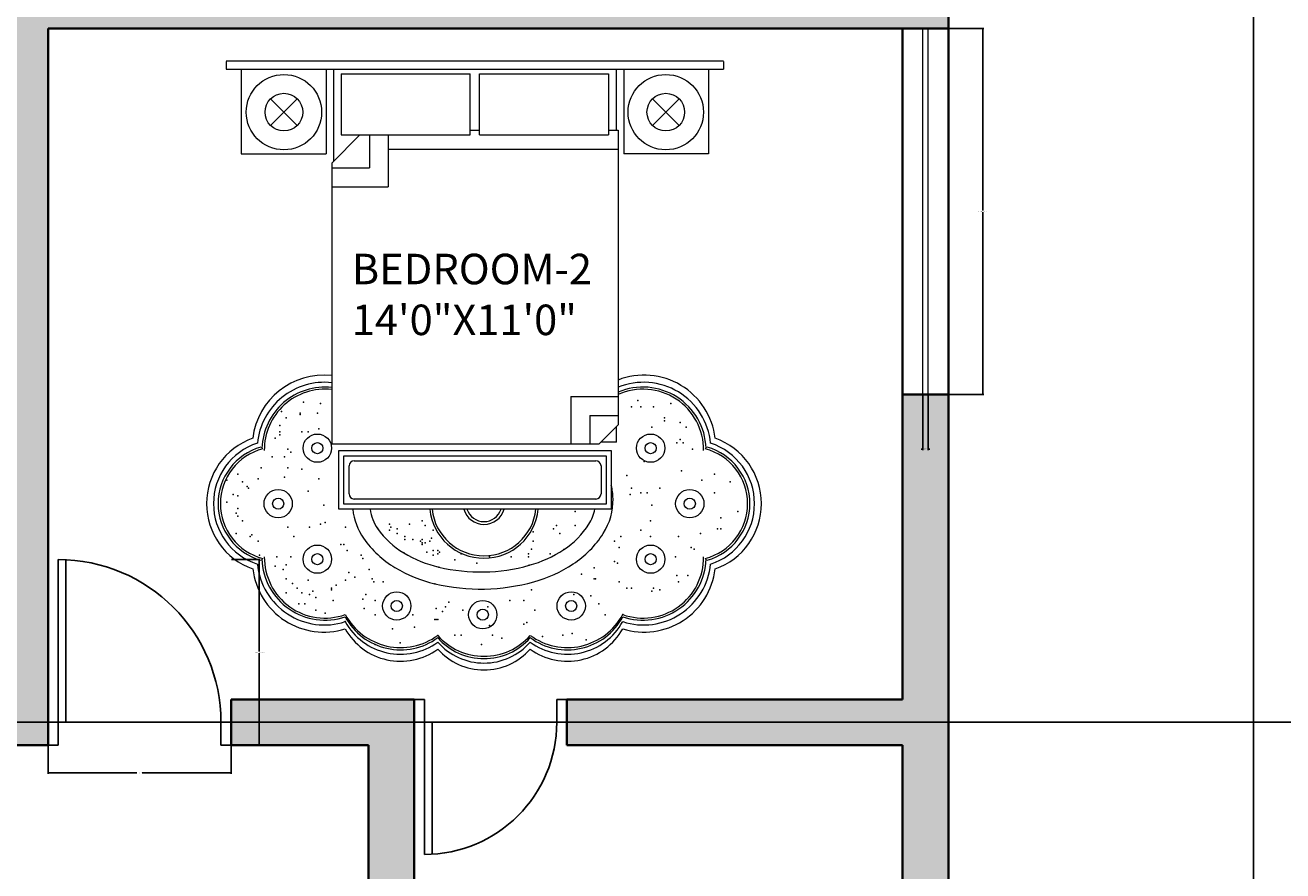
# Model space of a CAD drawing. Units: inches. Extents: x 5716 to 6907, y 12769 to 13594.
# Tile 9 of 17: x 6007 to 6254, y 13265 to 13432. Entities that reach past the tile are written whole.
import ezdxf

# ---------------------------------------------------------------- set-up
doc = ezdxf.new("R2010")
doc.units = ezdxf.units.IN
for name, color, linetype, lineweight in [('A-ANNO-DIMS', 2, 'Continuous', 18), ('A-AREA-IDEN', 7, 'Continuous', 18), ('A-DOOR', 4, 'Continuous', 25), ('A-FURN', 8, 'Continuous', 18), ('A-GLAZ', 4, 'Continuous', 18), ('A-WALL', 7, 'Continuous', 35), ('A-WALL-PATT', 252, 'Continuous', 13)]:
    doc.layers.add(name, color=color, linetype=linetype, lineweight=lineweight)
doc.styles.get("Standard").update_dxf_attribs({"font": 'arial.ttf'})
doc.dimstyles.get("Standard").update_dxf_attribs({"dimtxt": 0.18, "dimasz": 0.18, "dimexe": 0.18, "dimexo": 0.0625, "dimgap": 0.09, "dimtad": 0, "dimtih": 1, "dimtoh": 1, "dimdec": 4, "dimzin": 0, "dimdsep": 46, "dimtxsty": 'Standard', "dimcen": 0.09, "dimadec": 0, "dimazin": 0, "dimtfac": 1, "dimtdec": 4, "dimtofl": 0, "dimtmove": 0, "dimatfit": 3, "dimfxl": 1, "dimtolj": 1, "dimtzin": 0, "dimarcsym": 0})

# ---------------------------------------------------------------- blocks, each defined once
blk = doc.blocks.new('A$C1EC128A1')
for p, q in [((0.1147, 3.56), (3.0187, 3.56)), ((0.1147, 3.555), (0.1147, 3.511)), ((3.0187, 3.555), (3.0187, 3.511)), ((0.1147, 3.511), (3.0187, 3.511)), ((0.2027, 3.511), (0.2027, 3.4616)), ((0.2027, 3.4601), (0.2027, 3.016)), ((0.6977, 3.511), (0.6977, 3.016)), ((0.7417, 3.511), (0.7417, 2.972)), ((0.7857, 3.4835), (1.5392, 3.4835)), ((0.7857, 3.4835), (0.7857, 3.126)), ((1.5392, 3.126), (1.5392, 3.4835)), ((1.5942, 3.126), (1.5942, 3.4835)), ((1.5942, 3.4835), (2.3477, 3.4835)), ((2.3477, 3.4835), (2.3477, 3.126)), ((2.3917, 3.511), (2.3917, 3.1535)), ((2.4357, 3.511), (2.4357, 3.016)), ((2.9307, 3.511), (2.9307, 3.016)), ((0.3741, 3.1815), (0.5297, 3.337)), ((0.3741, 3.337), (0.5297, 3.1815)), ((2.6038, 3.337), (2.7594, 3.1815)), ((2.7594, 3.337), (2.6038, 3.1815)), ((0.7307, 2.961), (0.8957, 3.126)), ((0.7857, 3.126), (1.5392, 3.126)), ((0.9507, 3.126), (0.9507, 2.9335)), ((1.0607, 3.126), (1.0607, 2.8235)), ((1.5392, 3.1535), (1.5942, 3.1535)), ((1.5942, 3.126), (2.3477, 3.126)), ((2.3477, 3.1535), (2.4027, 3.1535)), ((2.4027, 3.1535), (2.4027, 1.432)), ((0.2027, 3.016), (0.6977, 3.016)), ((1.0607, 3.0435), (2.4027, 3.0435)), ((2.9307, 3.016), (2.4357, 3.016)), ((0.7307, 2.961), (0.7307, 1.322)), ((0.7307, 2.9335), (0.9507, 2.9335)), ((0.7307, 2.8235), (1.0607, 2.8235)), ((2.1277, 1.597), (2.4027, 1.597)), ((2.1277, 1.597), (2.1277, 1.322)), ((2.2377, 1.487), (2.2377, 1.322)), ((2.2377, 1.487), (2.4027, 1.487)), ((2.2927, 1.322), (2.4027, 1.432)), ((2.3917, 1.421), (2.3917, 1.333)), ((0.7307, 1.322), (2.2927, 1.322)), ((2.3037, 1.333), (2.3917, 1.333)), ((0.7721, 1.282), (2.3633, 1.282)), ((0.7721, 0.939), (0.7721, 1.282)), ((0.8021, 1.252), (2.3333, 1.252)), ((0.8021, 0.969), (0.8021, 1.252)), ((2.3333, 1.252), (2.3333, 0.969)), ((2.3633, 1.282), (2.3633, 0.939)), ((0.8321, 1.029), (0.8321, 1.192)), ((0.8621, 1.222), (2.2733, 1.222)), ((2.3033, 1.192), (2.3033, 1.029)), ((2.3333, 0.969), (0.8021, 0.969)), ((2.2733, 0.999), (0.8621, 0.999)), ((2.3633, 0.939), (0.7721, 0.939))]:
    blk.add_line(p, q)
for centre, radius in [((0.4519, 3.2593), 0.22), ((2.6816, 3.2593), 0.22), ((0.4519, 3.2593), 0.11), ((2.6816, 3.2593), 0.11), ((0.647, 1.2961), 0.0826), ((0.647, 1.2961), 0.0326), ((2.593, 1.2961), 0.0826), ((2.593, 1.2961), 0.0326), ((0.4183, 0.9718), 0.0826), ((2.8217, 0.9718), 0.0826), ((0.4183, 0.9718), 0.0326), ((2.8217, 0.9718), 0.0326), ((0.647, 0.6475), 0.0826), ((0.647, 0.6475), 0.0326), ((2.593, 0.6475), 0.0826), ((2.593, 0.6475), 0.0326), ((1.1109, 0.3741), 0.0826), ((2.1291, 0.3741), 0.0826), ((1.1109, 0.3741), 0.0326), ((1.6128, 0.3232), 0.0826), ((2.1291, 0.3741), 0.0326), ((1.6128, 0.3232), 0.0326)]:
    blk.add_circle(centre, radius)
for centre, radius, start, end in [((0.6854, 1.3045), 0.4183, 83.78243, 173.25148), ((2.5546, 1.3045), 0.4183, 6.74852, 111.27952), ((0.6884, 1.2877), 0.3932, 83.81567, 174.52996), ((0.6921, 1.2838), 0.369, 83.99709, 177.99757), ((0.6913, 1.2866), 0.3539, 83.60511, 180.66989), ((2.5516, 1.2877), 0.3932, 5.47004, 112.24899), ((2.5479, 1.2838), 0.369, 2.00243, 113.15364), ((2.5487, 1.2866), 0.3539, 359.33011, 114.35507), ((0.4048, 0.972), 0.4048, 109.45268, 180), ((0.4119, 0.972), 0.3714, 108.02557, 180), ((2.8281, 0.972), 0.3714, 0, 71.97443), ((2.8352, 0.972), 0.4048, 0, 70.54732), ((0.411, 0.972), 0.3435, 105.78906, 180), ((0.4122, 0.972), 0.3312, 104.76604, 180), ((2.8278, 0.972), 0.3312, 0, 75.23396), ((2.829, 0.972), 0.3435, 0, 74.21094), ((0.8621, 1.192), 0.03, 90, 180), ((2.2733, 1.192), 0.03, 0, 90), ((0.8621, 1.029), 0.03, 180, 270), ((2.2733, 1.029), 0.03, 270, 0), ((2.0084, 0.9935), 0.365, 1.17824, 13.48124), ((0.4048, 0.972), 0.4048, 180, 250.54732), ((0.4119, 0.972), 0.3714, 180, 251.97443), ((0.411, 0.972), 0.3435, 180, 254.21094), ((0.4122, 0.972), 0.3312, 180, 255.23396), ((2.0084, 0.9935), 0.365, 327.62391, 1.17824), ((2.8278, 0.972), 0.3312, 284.76604, 0), ((2.829, 0.972), 0.3435, 285.78906, 0), ((2.8281, 0.972), 0.3714, 288.02557, 0), ((2.8352, 0.972), 0.4048, 289.45268, 0), ((1.2169, 0.9773), 0.365, 186.01972, 214.73257), ((1.2169, 0.9773), 0.265, 188.30546, 214.73257), ((1.62, 0.972), 0.3185, 185.95071, 354.04929), ((1.62, 0.972), 0.305, 186.21512, 353.78488), ((1.62, 0.972), 0.1215, 195.7695, 344.2305), ((1.62, 0.972), 0.105, 198.32909, 341.67091), ((2.0084, 0.9935), 0.265, 327.62391, 348.11864), ((1.4035, 1.1066), 0.492, 214.73257, 239.1926), ((1.8167, 1.1151), 0.492, 303.16388, 327.62391), ((1.4035, 1.1066), 0.592, 214.73257, 239.1926), ((1.8167, 1.1151), 0.592, 303.16388, 327.62391), ((0.6913, 0.6574), 0.3539, 179.33011, 289.59453), ((1.5241, 1.3089), 0.7275, 239.1926, 256.67462), ((1.6878, 1.3123), 0.7275, 285.68186, 303.16388), ((2.5487, 0.6574), 0.3539, 250.40547, 0.66989), ((0.6854, 0.6395), 0.4183, 186.74852, 287.32326), ((0.6884, 0.6563), 0.3932, 185.47004, 288.01752), ((0.6921, 0.6602), 0.369, 182.00243, 288.62304), ((1.5241, 1.3089), 0.8275, 239.1926, 256.67462), ((1.5995, 1.627), 1.0544, 256.67462, 271.17824), ((1.5995, 1.627), 1.0544, 271.17824, 285.68186), ((1.6878, 1.3123), 0.8275, 285.68186, 303.16388), ((2.5479, 0.6602), 0.369, 251.37696, 357.99757), ((2.5516, 0.6563), 0.3932, 251.98248, 354.52996), ((2.5546, 0.6395), 0.4183, 252.67674, 353.25148), ((1.5995, 1.627), 1.1544, 271.17824, 285.68186), ((1.5995, 1.627), 1.1544, 256.67462, 271.17824), ((1.1328, 0.4977), 0.3665, 208.29135, 306.34788), ((1.1328, 0.4842), 0.3665, 208.29135, 306.34788), ((2.1072, 0.4977), 0.3665, 233.65212, 331.70865), ((2.1072, 0.4842), 0.3665, 233.65212, 331.70865), ((1.133, 0.4609), 0.369, 208.93019, 306.02618), ((1.1324, 0.4204), 0.3694, 209.22014, 306.07902), ((2.107, 0.4609), 0.369, 233.97382, 331.06981), ((2.1076, 0.4204), 0.3694, 233.92098, 330.77986), ((1.6145, 0.4295), 0.3486, 220.6393, 270.90521), ((1.6145, 0.416), 0.3486, 220.6393, 270.90521), ((1.62, 0.4004), 0.3599, 221.38778, 270), ((1.6255, 0.4295), 0.3486, 269.09479, 319.3607), ((1.6255, 0.416), 0.3486, 269.09479, 319.3607), ((1.62, 0.4004), 0.3599, 270, 318.61222), ((1.62, 0.36), 0.36, 221.41854, 270), ((1.62, 0.36), 0.36, 270, 318.58146)]:
    blk.add_arc(centre, radius, start, end)
for p in [(0.5654, 1.5652), (0.6657, 1.5561), (2.5184, 1.5744), (2.71, 1.5561), (0.4376, 1.5104), (0.465, 1.4739), (0.5471, 1.5013), (0.5471, 1.4922), (0.6475, 1.5013), (2.4819, 1.5378), (2.5366, 1.5378), (2.6097, 1.5378), (2.6735, 1.4739), (0.4285, 1.4282), (0.6566, 1.41), (2.6005, 1.4191), (2.6735, 1.4556), (2.7648, 1.4465), (2.8013, 1.4191), (0.4011, 1.3552), (0.4285, 1.3917), (0.4285, 1.3734), (0.5562, 1.3917), (0.5927, 1.3917), (2.3917, 1.333), (2.7465, 1.3278), (2.7648, 1.346), (2.7831, 1.3278), (0.4741, 1.2912), (0.4923, 1.273), (2.8378, 1.2912), (0.3189, 1.1816), (0.3828, 1.2456), (0.4558, 1.2456), (0.4741, 1.1816), (2.5549, 1.2182), (0.1182, 1.1085), (0.1821, 1.1451), (0.3007, 1.1177), (0.4558, 1.1268), (0.5562, 1.1725), (0.6566, 1.1177), (2.4545, 1.1359), (2.7739, 1.1634), (2.8926, 1.1085), (2.9656, 1.1451), (0.2094, 1.0994), (0.2368, 1.072), (0.2459, 1.0629), (0.5927, 1.0446), (2.4819, 1.0629), (2.5366, 1.0355), (2.5731, 1.0355), (2.6462, 1.0629), (2.9656, 1.0355), (3.0568, 1.0994), (0.1182, 0.9807), (0.1547, 1.0263), (0.1821, 1.0172), (0.684, 0.9624), (2.4728, 1.0263), (2.6005, 0.9624), (0.1729, 0.9167), (0.1821, 0.9441), (0.1821, 0.8985), (1.3032, 0.939), (1.3168, 0.939), (2.1533, 0.9259), (3.0021, 0.8893), (3.1025, 0.9259), (0.2094, 0.8711), (0.4741, 0.8345), (0.6019, 0.8345), (0.6657, 0.8528), (0.6931, 0.8619), (0.8118, 0.8345), (0.9992, 0.8263), (1.0673, 0.8528), (1.0673, 0.8163), (1.0764, 0.8345), (1.1129, 0.8254), (1.1859, 0.8528), (1.259, 0.8711), (1.2772, 0.8437), (1.3228, 0.8163), (2.0256, 0.8254), (2.0438, 0.8437), (2.0438, 0.8437), (2.1533, 0.8437), (2.5366, 0.8163), (2.5914, 0.8711), (2.9838, 0.8254), (3.0021, 0.8254), (0.1729, 0.798), (0.2551, 0.7797), (0.2642, 0.7889), (0.3007, 0.7523), (0.5106, 0.7797), (1.1129, 0.798), (1.1586, 0.7797), (1.1586, 0.7615), (1.2042, 0.7615), (1.2498, 0.7523), (1.259, 0.7615), (1.259, 0.7432), (1.2772, 0.7432), (1.3046, 0.7523), (1.3137, 0.7706), (1.9069, 0.8071), (1.9069, 0.7523), (2.0621, 0.798), (2.3815, 0.7523), (2.418, 0.7797), (2.5914, 0.7797), (2.7557, 0.7797), (2.8834, 0.798), (0.3098, 0.6701), (0.4102, 0.661), (0.4923, 0.661), (0.7844, 0.7341), (0.8026, 0.7341), (0.8209, 0.6975), (0.903, 0.6701), (1.1515, 0.684), (1.1515, 0.684), (1.1515, 0.684), (1.259, 0.7341), (1.2863, 0.6884), (1.3228, 0.6975), (1.3228, 0.6701), (1.3502, 0.6975), (1.3502, 0.6793), (1.3593, 0.6884), (1.4871, 0.6793), (1.6514, 0.661), (1.6514, 0.661), (1.7792, 0.661), (1.8795, 0.6793), (1.8795, 0.661), (1.8978, 0.7067), (2.0073, 0.6793), (2.0858, 0.7033), (2.4089, 0.7158), (2.7374, 0.661), (2.8287, 0.7158), (2.8469, 0.7067), (0.4011, 0.6062), (0.4467, 0.5879), (0.465, 0.6153), (0.9122, 0.6519), (0.9487, 0.5879), (1.3564, 0.601), (1.4506, 0.6427), (1.5784, 0.6245), (1.8845, 0.6118), (2.2629, 0.597), (2.3815, 0.6336), (2.3997, 0.6245), (0.465, 0.5331), (0.5927, 0.524), (0.8118, 0.524), (0.83, 0.5696), (0.8665, 0.5422), (0.9669, 0.5331), (0.976, 0.5148), (1.0308, 0.5148), (2.1898, 0.5605), (2.2629, 0.5331), (2.272, 0.5331), (2.4089, 0.5148), (2.7465, 0.5514), (2.7557, 0.5148), (2.8104, 0.5514), (0.465, 0.4509), (0.5015, 0.5057), (0.5289, 0.4783), (0.5562, 0.4509), (0.6019, 0.4418), (0.6201, 0.46), (0.7296, 0.4783), (0.7296, 0.4692), (0.757, 0.4966), (0.9304, 0.4418), (1.3334, 0.5037), (1.8978, 0.4692), (2.1442, 0.4418), (2.4545, 0.4783), (2.4819, 0.4783), (2.6005, 0.46), (2.6097, 0.4783), (2.6462, 0.4692), (0.538, 0.387), (0.5745, 0.387), (0.6384, 0.4235), (0.7388, 0.4052), (0.7388, 0.4052), (0.9122, 0.4144), (0.9852, 0.4052), (1.3959, 0.3687), (1.4141, 0.3961), (1.6423, 0.3687), (1.77, 0.4052), (1.8522, 0.4052), (2.2446, 0.4326), (2.2902, 0.387), (0.6384, 0.3504), (0.6931, 0.3322), (0.9213, 0.3596), (0.9852, 0.323), (1.2042, 0.323), (1.332, 0.2956), (1.3411, 0.3596), (1.3411, 0.2956), (1.3502, 0.2956), (1.3776, 0.3413), (1.4962, 0.3504), (1.9161, 0.3504), (2.3267, 0.323), (2.43, 0.324), (0.81, 0.2824), (1.0856, 0.2408), (1.2133, 0.25), (1.6514, 0.2591), (1.8522, 0.2682), (1.8704, 0.2774), (0.9852, 0.1495), (1.1312, 0.1586), (1.35, 0.2025), (1.4506, 0.2043), (1.4871, 0.2043), (1.6058, 0.1495), (1.6696, 0.2043), (1.7244, 0.186), (1.9617, 0.1952), (2.0803, 0.2043), (2.1351, 0.2134), (2.2172, 0.1769)]:
    blk.add_point(p)
blk = doc.blocks.new('DOOR-SWING-30IN')
for p, q in [((0, 4.5), (-2, 4.5)), ((0, 0), (0, 4.5)), ((26, 0), (26, 4.5)), ((26, 4.5), (28, 4.5)), ((-2, 0), (0, 0)), ((0, -26), (0, 0)), ((0, 0), (1.5, 0)), ((1.5, -25.96), (1.5, 0)), ((28, 0), (26, 0))]:
    blk.add_line(p, q)
blk.add_arc((0, 0), 26, 270, 0)
blk = doc.blocks.new('DOOR-SWING-36IN')
for p, q in [((0, 32), (0, 0)), ((1.5, 31.96), (1.5, 0)), ((-2, 0), (0, 0)), ((0, 0), (0, -4.5)), ((0, 0), (1.5, 0)), ((34, 0), (32, 0)), ((32, 0), (32, -4.5)), ((0, -4.5), (-2, -4.5)), ((32, -4.5), (34, -4.5))]:
    blk.add_line(p, q)
blk.add_arc((0, 0), 32, 0, 90)
blk = doc.blocks.new('WIN-GLAZING-72IN')
for p, q in [((0, 0), (0, -72)), ((1, 0), (1, -72))]:
    blk.add_line(p, q)
blk = doc.blocks.new('*D23')
at = {"layer": 'A-ANNO-DIMS', "color": 0, "lineweight": -2, "transparency": 16777216}
for p, q in [((6047.09, 13326.65), (6052.68, 13326.65)), ((6052.5, 13326.47), (6052.5, 13308.58)), ((6052.5, 13290.33), (6052.5, 13308.22)), ((6047.09, 13290.15), (6052.68, 13290.15))]:
    blk.add_line(p, q, dxfattribs=at)
at = {"layer": 'A-ANNO-DIMS', "color": 0, "transparency": 16777216}
for points in [[(6052.47, 13326.47), (6052.53, 13326.47), (6052.5, 13326.65)], [(6052.47, 13290.33), (6052.53, 13290.33), (6052.5, 13290.15)]]:
    blk.add_solid(points, dxfattribs=at)
at = {"layer": 'Defpoints', "color": 0, "transparency": 16777216}
for p in [(6047.02, 13326.65), (6052.5, 13326.65), (6047.02, 13290.15)]:
    blk.add_point(p, dxfattribs=at)
at = {"layer": 'A-ANNO-DIMS', "color": 0, "transparency": 16777216, "insert": (6052.5, 13308.4), "char_height": 0.18, "attachment_point": 5}
blk.add_mtext('\\A1;ROOM DOOR 37 TYP.', dxfattribs=at)
blk = doc.blocks.new('*D24')
at = {"layer": 'A-ANNO-DIMS', "color": 0, "lineweight": -2, "transparency": 16777216}
for p, q in [((6011.02, 13290.09), (6011.02, 13284.49)), ((6047.02, 13290.09), (6047.02, 13284.49)), ((6011.2, 13284.67), (6028.49, 13284.67)), ((6046.84, 13284.67), (6029.55, 13284.67))]:
    blk.add_line(p, q, dxfattribs=at)
at = {"layer": 'A-ANNO-DIMS', "color": 0, "transparency": 16777216}
for points in [[(6011.2, 13284.7), (6011.2, 13284.64), (6011.02, 13284.67)], [(6046.84, 13284.7), (6046.84, 13284.64), (6047.02, 13284.67)]]:
    blk.add_solid(points, dxfattribs=at)
at = {"layer": 'Defpoints', "color": 0, "transparency": 16777216}
for p in [(6011.02, 13290.15), (6047.02, 13290.15), (6047.02, 13284.67)]:
    blk.add_point(p, dxfattribs=at)
at = {"layer": 'A-ANNO-DIMS', "color": 0, "transparency": 16777216, "insert": (6029.02, 13284.67), "char_height": 0.18, "attachment_point": 5}
blk.add_mtext('\\A1;36 TYP.', dxfattribs=at)
blk = doc.blocks.new('*D25')
at = {"layer": 'A-ANNO-DIMS', "color": 0, "lineweight": -2, "transparency": 16777216}
for p, q in [((6184.09, 13431.15), (6195, 13431.15)), ((6194.82, 13430.97), (6194.82, 13395.33)), ((6194.82, 13359.33), (6194.82, 13394.97)), ((6184.09, 13359.15), (6195, 13359.15))]:
    blk.add_line(p, q, dxfattribs=at)
at = {"layer": 'A-ANNO-DIMS', "color": 0, "transparency": 16777216}
for points in [[(6194.79, 13430.97), (6194.85, 13430.97), (6194.82, 13431.15)], [(6194.79, 13359.33), (6194.85, 13359.33), (6194.82, 13359.15)]]:
    blk.add_solid(points, dxfattribs=at)
at = {"layer": 'Defpoints', "color": 0, "transparency": 16777216}
for p in [(6184.02, 13431.15), (6184.02, 13359.15), (6194.82, 13359.15)]:
    blk.add_point(p, dxfattribs=at)
at = {"layer": 'A-ANNO-DIMS', "color": 0, "transparency": 16777216, "insert": (6194.82, 13395.15), "char_height": 0.18, "attachment_point": 5}
blk.add_mtext('\\A1;WINDOW 72 TYP.', dxfattribs=at)
blk = doc.blocks.new('*D26')
at = {"layer": 'A-ANNO-DIMS', "color": 0, "lineweight": -2, "transparency": 16777216}
for p, q in [((6183.02, 13359.09), (6183.02, 13348.17)), ((6184.02, 13359.09), (6184.02, 13348.17)), ((6182.84, 13348.35), (6182.66, 13348.35)), ((6184.2, 13348.35), (6184.38, 13348.35))]:
    blk.add_line(p, q, dxfattribs=at)
at = {"layer": 'A-ANNO-DIMS', "color": 0, "transparency": 16777216}
for points in [[(6182.84, 13348.38), (6182.84, 13348.32), (6183.02, 13348.35)], [(6184.2, 13348.38), (6184.2, 13348.32), (6184.02, 13348.35)]]:
    blk.add_solid(points, dxfattribs=at)
at = {"layer": 'Defpoints', "color": 0, "transparency": 16777216}
for p in [(6183.02, 13359.15), (6184.02, 13359.15), (6183.02, 13348.35)]:
    blk.add_point(p, dxfattribs=at)
at = {"layer": 'A-ANNO-DIMS', "color": 0, "transparency": 16777216, "insert": (6183.52, 13348.35), "char_height": 0.18, "attachment_point": 5}
blk.add_mtext('\\A1;1 TYP.', dxfattribs=at)
blk = doc.blocks.new('*D51')
at = {"layer": 'A-ANNO-DIMS', "color": 0, "lineweight": -2, "transparency": 16777216}
for p, q in [((5819.02, 13440.21), (5819.02, 13594.38)), ((5819.2, 13594.2), (6033.23, 13594.2)), ((6247.84, 13594.2), (6033.82, 13594.2)), ((6248.02, 13194.21), (6248.02, 13594.38))]:
    blk.add_line(p, q, dxfattribs=at)
at = {"layer": 'A-ANNO-DIMS', "color": 0, "transparency": 16777216}
for points in [[(5819.2, 13594.23), (5819.2, 13594.17), (5819.02, 13594.2)], [(6247.84, 13594.23), (6247.84, 13594.17), (6248.02, 13594.2)]]:
    blk.add_solid(points, dxfattribs=at)
at = {"layer": 'Defpoints', "color": 0, "transparency": 16777216}
for p in [(6248.02, 13594.2), (5819.02, 13440.15), (6248.02, 13194.15)]:
    blk.add_point(p, dxfattribs=at)
at = {"layer": 'A-ANNO-DIMS', "color": 0, "transparency": 16777216, "insert": (6033.52, 13594.2), "char_height": 0.18, "attachment_point": 5}
blk.add_mtext('\\A1;429', dxfattribs=at)
blk = doc.blocks.new('*D52')
at = {"layer": 'A-ANNO-DIMS', "color": 0, "lineweight": -2, "transparency": 16777216}
for p, q in [((6267.34, 13440.15), (5716.04, 13440.15)), ((5716.22, 13439.97), (5716.22, 13140.83)), ((5716.22, 12841.33), (5716.22, 13140.47)), ((6267.34, 12841.15), (5716.04, 12841.15))]:
    blk.add_line(p, q, dxfattribs=at)
at = {"layer": 'A-ANNO-DIMS', "color": 0, "transparency": 16777216}
for points in [[(5716.19, 13439.97), (5716.25, 13439.97), (5716.22, 13440.15)], [(5716.19, 12841.33), (5716.25, 12841.33), (5716.22, 12841.15)]]:
    blk.add_solid(points, dxfattribs=at)
at = {"layer": 'Defpoints', "color": 0, "transparency": 16777216}
for p in [(6267.41, 13440.15), (5716.22, 12841.15), (6267.41, 12841.15)]:
    blk.add_point(p, dxfattribs=at)
at = {"layer": 'A-ANNO-DIMS', "color": 0, "transparency": 16777216, "insert": (5716.22, 13140.65), "char_height": 0.18, "attachment_point": 5}
blk.add_mtext('\\A1;599', dxfattribs=at)
blk = doc.blocks.new('*D58')
at = {"layer": 'A-ANNO-DIMS', "color": 0, "lineweight": -2, "transparency": 16777216}
for p, q in [((6736.67, 13435.65), (5716.04, 13435.65)), ((5716.22, 13435.47), (5716.22, 13365.33)), ((5716.22, 13294.83), (5716.22, 13364.97)), ((6736.67, 13294.65), (5716.04, 13294.65))]:
    blk.add_line(p, q, dxfattribs=at)
at = {"layer": 'A-ANNO-DIMS', "color": 0, "transparency": 16777216}
for points in [[(5716.19, 13435.47), (5716.25, 13435.47), (5716.22, 13435.65)], [(5716.19, 13294.83), (5716.25, 13294.83), (5716.22, 13294.65)]]:
    blk.add_solid(points, dxfattribs=at)
at = {"layer": 'Defpoints', "color": 0, "transparency": 16777216}
for p in [(6736.73, 13435.65), (5716.22, 13294.65), (6736.73, 13294.65)]:
    blk.add_point(p, dxfattribs=at)
at = {"layer": 'A-ANNO-DIMS', "color": 0, "transparency": 16777216, "insert": (5716.22, 13365.15), "char_height": 0.18, "attachment_point": 5}
blk.add_mtext('\\A1;141', dxfattribs=at)
blk = doc.blocks.new('*D59')
at = {"layer": 'A-ANNO-DIMS', "color": 0, "lineweight": -2, "transparency": 16777216}
for p, q in [((6736.67, 13294.65), (5716.04, 13294.65)), ((5716.22, 13294.47), (5716.22, 13248.33)), ((5716.22, 13201.83), (5716.22, 13247.97)), ((6736.67, 13201.65), (5716.04, 13201.65))]:
    blk.add_line(p, q, dxfattribs=at)
at = {"layer": 'A-ANNO-DIMS', "color": 0, "transparency": 16777216}
for points in [[(5716.19, 13294.47), (5716.25, 13294.47), (5716.22, 13294.65)], [(5716.19, 13201.83), (5716.25, 13201.83), (5716.22, 13201.65)]]:
    blk.add_solid(points, dxfattribs=at)
at = {"layer": 'Defpoints', "color": 0, "transparency": 16777216}
for p in [(6736.73, 13294.65), (5716.22, 13201.65), (6736.73, 13201.65)]:
    blk.add_point(p, dxfattribs=at)
at = {"layer": 'A-ANNO-DIMS', "color": 0, "transparency": 16777216, "insert": (5716.22, 13248.15), "char_height": 0.18, "attachment_point": 5}
blk.add_mtext('\\A1;93', dxfattribs=at)

msp = doc.modelspace()

# ---------------------------------------------------------------- hatches: boundary and pattern name
at = {"layer": 'A-WALL-PATT'}
h = msp.add_hatch(color=256, dxfattribs=at)
h.dxf.hatch_style = 1
h.paths.add_polyline_path([(6188.02, 13440.15), (5819.02, 13440.15), (5819.02, 13431.15), (6002.02, 13431.15), (6002.02, 13290.15), (6011.02, 13290.15), (6011.02, 13431.15), (6188.02, 13431.15)])
h = msp.add_hatch(color=256, dxfattribs=at)
h.dxf.hatch_style = 1
h.paths.add_polyline_path([(6188.02, 13359.15), (6179.02, 13359.15), (6179.02, 13299.15), (6113.02, 13299.15), (6113.02, 13290.15), (6179.02, 13290.15), (6179.02, 13254.15), (6188.02, 13254.15)])
h = msp.add_hatch(color=256, dxfattribs=at)
h.dxf.hatch_style = 1
h.paths.add_polyline_path([(6188.02, 13230.15), (6179.02, 13230.15), (6179.02, 13194.15), (6083.02, 13194.15), (6083.02, 13299.15), (6047.02, 13299.15), (6047.02, 13290.15), (6074.02, 13290.15), (6074.02, 13185.15), (6188.02, 13185.15)])

# ---------------------------------------------------------------- linework, layer by layer
at = {"layer": 'A-WALL'}
for p, q in [((6188.02, 13440.15), (6188.02, 13185.15)), ((6011.02, 13431.15), (6011.02, 13290.15)), ((6011.02, 13431.15), (6188.02, 13431.15)), ((6179.02, 13431.15), (6179.02, 13299.15)), ((6179.02, 13359.15), (6188.02, 13359.15)), ((6047.02, 13299.15), (6083.02, 13299.15)), ((6047.02, 13299.15), (6047.02, 13290.15)), ((6083.02, 13299.15), (6083.02, 13194.15)), ((6113.02, 13299.15), (6113.02, 13290.15)), ((6113.02, 13299.15), (6179.02, 13299.15)), ((6002.02, 13290.15), (6011.02, 13290.15)), ((6047.02, 13290.15), (6074.02, 13290.15)), ((6074.02, 13290.15), (6074.02, 13185.15)), ((6113.02, 13290.15), (6179.02, 13290.15)), ((6179.02, 13290.15), (6179.02, 13194.15))]:
    msp.add_line(p, q, dxfattribs=at)

# ---------------------------------------------------------------- block references
at = {"layer": 'A-DOOR'}
for name, p in [('DOOR-SWING-36IN', (6013.02, 13294.65)), ('DOOR-SWING-30IN', (6085.02, 13294.65))]:
    msp.add_blockref(name, p, dxfattribs=at)
at = {"layer": 'A-FURN', "xscale": 33.66910864864256, "yscale": 33.66910864864256, "zscale": 33.66910864864256}
msp.add_blockref('A$C1EC128A1', (6042.18, 13304.93), dxfattribs=at)
at = {"layer": 'A-GLAZ', "rotation": 180}
msp.add_blockref('WIN-GLAZING-72IN', (6184.02, 13359.15), dxfattribs=at)

# ---------------------------------------------------------------- texts
at = {"layer": 'A-AREA-IDEN', "insert": (6070.74, 13386.81), "char_height": 6, "attachment_point": 1}
msp.add_mtext_dynamic_manual_height_columns('BEDROOM-2\\P14\'0"X11\'0"', width=94.1172, gutter_width=12.5, heights=[0], dxfattribs=at)

# ---------------------------------------------------------------- dimensions: what is measured, and where the dimension line sits
at = {"layer": 'A-ANNO-DIMS'}
dim = msp.add_linear_dim(base=(6248.02, 13594.2), p1=(5819.02, 13440.15), p2=(6248.02, 13194.15), dimstyle='Standard', override={"dimdec": 0, "dimlfac": 1, "dimrnd": 0, "dimzin": 0, "dimdsep": 46, "dimlunit": 2}, dxfattribs=at)
dim.commit()
dim.dimension.update_dxf_attribs({"geometry": '*D51', "text_midpoint": (6033.52, 13594.2)})
for base, p1, p2, picture, middle in [((5716.22, 12841.15), (6267.41, 13440.15), (6267.41, 12841.15), '*D52', (5716.22, 13140.65)), ((5716.22, 13294.65), (6736.73, 13435.65), (6736.73, 13294.65), '*D58', (5716.22, 13365.15)), ((5716.22, 13201.65), (6736.73, 13294.65), (6736.73, 13201.65), '*D59', (5716.22, 13248.15))]:
    dim = msp.add_linear_dim(base=base, p1=p1, p2=p2, angle=90, dimstyle='Standard', override={"dimdec": 0, "dimlfac": 1, "dimrnd": 0, "dimzin": 0, "dimdsep": 46, "dimlunit": 2}, dxfattribs=at)
    dim.commit()
    dim.dimension.update_dxf_attribs({"geometry": picture, "text_midpoint": middle})
for base, p1, p2, angle, text, picture, middle in [((6194.82, 13359.15), (6184.02, 13431.15), (6184.02, 13359.15), 270, 'WINDOW <> TYP.', '*D25', (6194.82, 13395.15)), ((6183.02, 13348.35), (6184.02, 13359.15), (6183.02, 13359.15), 180, '<> TYP.', '*D26', (6183.52, 13348.35)), ((6052.49751723, 13326.64894948), (6047.02251723, 13290.14894948), (6047.02251723, 13326.64894948), 90, 'ROOM DOOR <> TYP.', '*D23', (6052.49751723, 13308.39894948))]:
    dim = msp.add_linear_dim(base=base, p1=p1, p2=p2, angle=angle, text=text, dimstyle='Standard', override={"dimdec": 0, "dimlfac": 1, "dimrnd": 0, "dimzin": 0, "dimdsep": 46, "dimlunit": 2}, dxfattribs=at)
    dim.commit()
    dim.dimension.update_dxf_attribs({"geometry": picture, "text_midpoint": middle})
dim = msp.add_linear_dim(base=(6047.02, 13284.67), p1=(6011.02, 13290.15), p2=(6047.02, 13290.15), text='<> TYP.', dimstyle='Standard', override={"dimdec": 0, "dimlfac": 1, "dimrnd": 0, "dimzin": 0, "dimdsep": 46, "dimlunit": 2}, dxfattribs=at)
dim.commit()
dim.dimension.update_dxf_attribs({"geometry": '*D24', "text_midpoint": (6029.02, 13284.67)})

doc.saveas('drawing.dxf')
